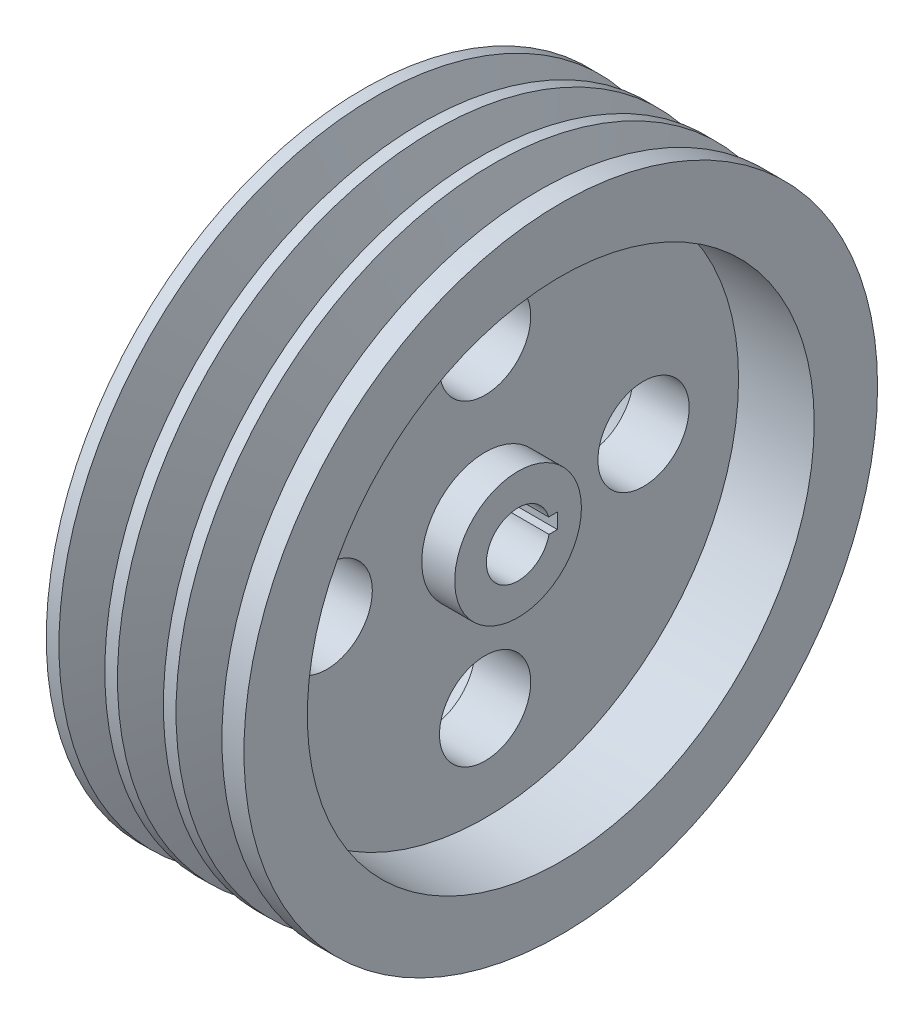
ISO-10303-21;
HEADER;
FILE_DESCRIPTION(('STEP AP214'),'2;1');
FILE_NAME('part.step','',(''),(''),'','','');
FILE_SCHEMA(('AUTOMOTIVE_DESIGN { 1 0 10303 214 1 1 1 1 }'));
ENDSEC;
DATA;
#1=APPLICATION_CONTEXT('core data for automotive mechanical design processes');
#2=APPLICATION_PROTOCOL_DEFINITION('international standard','automotive_design',2000,#1);
#3=PRODUCT_CONTEXT('',#1,'mechanical');
#4=PRODUCT('Part','Part','',(#3));
#5=PRODUCT_RELATED_PRODUCT_CATEGORY('part','',(#4));
#6=PRODUCT_DEFINITION_FORMATION('','',#4);
#7=PRODUCT_DEFINITION_CONTEXT('part definition',#1,'design');
#8=PRODUCT_DEFINITION('design','',#6,#7);
#9=PRODUCT_DEFINITION_SHAPE('','',#8);
#10=(LENGTH_UNIT() NAMED_UNIT(*) SI_UNIT(.MILLI.,.METRE.));
#11=(NAMED_UNIT(*) PLANE_ANGLE_UNIT() SI_UNIT($,.RADIAN.));
#12=(NAMED_UNIT(*) SI_UNIT($,.STERADIAN.) SOLID_ANGLE_UNIT());
#13=UNCERTAINTY_MEASURE_WITH_UNIT(LENGTH_MEASURE(1.E-05),#10,'distance_accuracy_value','');
#14=(GEOMETRIC_REPRESENTATION_CONTEXT(3) GLOBAL_UNCERTAINTY_ASSIGNED_CONTEXT((#13)) GLOBAL_UNIT_ASSIGNED_CONTEXT((#10,
#11,#12)) REPRESENTATION_CONTEXT('',''));
#15=CARTESIAN_POINT('',(0.,0.,0.));
#16=DIRECTION('',(0.,0.,1.));
#17=DIRECTION('',(1.,0.,0.));
#18=AXIS2_PLACEMENT_3D('',#15,#16,#17);
#19=CARTESIAN_POINT('',(-24.,0.,0.));
#20=DIRECTION('',(1.,0.,0.));
#21=DIRECTION('',(0.,0.,-1.));
#22=AXIS2_PLACEMENT_3D('',#19,#20,#21);
#23=PLANE('',#22);
#24=CARTESIAN_POINT('',(-24.,0.,0.));
#25=DIRECTION('',(1.,0.,0.));
#26=DIRECTION('',(0.,0.,-1.));
#27=AXIS2_PLACEMENT_3D('',#24,#25,#26);
#28=CIRCLE('',#27,25.);
#29=CARTESIAN_POINT('',(-24.,0.,-25.));
#30=VERTEX_POINT('',#29);
#31=EDGE_CURVE('E107',#30,#30,#28,.T.);
#32=ORIENTED_EDGE('',*,*,#31,.F.);
#33=EDGE_LOOP('',(#32));
#34=FACE_BOUND('',#33,.T.);
#35=DIRECTION('',(0.,0.,-1.));
#36=VECTOR('',#35,1.);
#37=CARTESIAN_POINT('',(-24.,3.31611385733775,0.));
#38=LINE('',#37,#36);
#39=CARTESIAN_POINT('',(-24.,3.31611385733775,-12.0521113870215));
#40=VERTEX_POINT('',#39);
#41=CARTESIAN_POINT('',(-24.,3.31611385733775,-15.5));
#42=VERTEX_POINT('',#41);
#43=EDGE_CURVE('E105',#40,#42,#38,.T.);
#44=ORIENTED_EDGE('',*,*,#43,.F.);
#45=CARTESIAN_POINT('',(-24.,0.,0.));
#46=DIRECTION('',(1.,0.,0.));
#47=DIRECTION('',(0.,0.,-1.));
#48=AXIS2_PLACEMENT_3D('',#45,#46,#47);
#49=CIRCLE('',#48,12.5);
#50=CARTESIAN_POINT('',(-24.,-2.68388614266225,-12.2084706320335));
#51=VERTEX_POINT('',#50);
#52=EDGE_CURVE('E95',#40,#51,#49,.T.);
#53=ORIENTED_EDGE('',*,*,#52,.T.);
#54=DIRECTION('',(0.,0.,-1.));
#55=VECTOR('',#54,1.);
#56=CARTESIAN_POINT('',(-24.,-2.68388614266225,0.));
#57=LINE('',#56,#55);
#58=CARTESIAN_POINT('',(-24.,-2.68388614266225,-15.5));
#59=VERTEX_POINT('',#58);
#60=EDGE_CURVE('E100',#51,#59,#57,.T.);
#61=ORIENTED_EDGE('',*,*,#60,.T.);
#62=DIRECTION('',(0.,-1.,0.));
#63=VECTOR('',#62,1.);
#64=CARTESIAN_POINT('',(-24.,0.,-15.5));
#65=LINE('',#64,#63);
#66=EDGE_CURVE('E110',#42,#59,#65,.T.);
#67=ORIENTED_EDGE('',*,*,#66,.F.);
#68=EDGE_LOOP('',(#44,#53,#61,#67));
#69=FACE_BOUND('',#68,.T.);
#70=ADVANCED_FACE('F53',(#34,#69),#23,.F.);
#71=CARTESIAN_POINT('',(24.,0.,0.));
#72=DIRECTION('',(1.,0.,0.));
#73=DIRECTION('',(0.,0.,-1.));
#74=AXIS2_PLACEMENT_3D('',#71,#72,#73);
#75=PLANE('',#74);
#76=CARTESIAN_POINT('',(24.,0.,0.));
#77=DIRECTION('',(1.,0.,0.));
#78=DIRECTION('',(0.,0.,-1.));
#79=AXIS2_PLACEMENT_3D('',#76,#77,#78);
#80=CIRCLE('',#79,25.);
#81=CARTESIAN_POINT('',(24.,0.,-25.));
#82=VERTEX_POINT('',#81);
#83=EDGE_CURVE('E112',#82,#82,#80,.T.);
#84=ORIENTED_EDGE('',*,*,#83,.T.);
#85=EDGE_LOOP('',(#84));
#86=FACE_BOUND('',#85,.T.);
#87=CARTESIAN_POINT('',(24.,0.,0.));
#88=DIRECTION('',(1.,0.,0.));
#89=DIRECTION('',(0.,0.,-1.));
#90=AXIS2_PLACEMENT_3D('',#87,#88,#89);
#91=CIRCLE('',#90,12.5);
#92=CARTESIAN_POINT('',(24.,3.31611385733775,-12.0521113870215));
#93=VERTEX_POINT('',#92);
#94=CARTESIAN_POINT('',(24.,-2.68388614266225,-12.2084706320335));
#95=VERTEX_POINT('',#94);
#96=EDGE_CURVE('E189',#93,#95,#91,.T.);
#97=ORIENTED_EDGE('',*,*,#96,.F.);
#98=DIRECTION('',(0.,0.,-1.));
#99=VECTOR('',#98,1.);
#100=CARTESIAN_POINT('',(24.,3.31611385733775,0.));
#101=LINE('',#100,#99);
#102=CARTESIAN_POINT('',(24.,3.31611385733775,-15.5));
#103=VERTEX_POINT('',#102);
#104=EDGE_CURVE('E12',#93,#103,#101,.T.);
#105=ORIENTED_EDGE('',*,*,#104,.T.);
#106=DIRECTION('',(0.,-1.,0.));
#107=VECTOR('',#106,1.);
#108=CARTESIAN_POINT('',(24.,0.,-15.5));
#109=LINE('',#108,#107);
#110=CARTESIAN_POINT('',(24.,-2.68388614266225,-15.5));
#111=VERTEX_POINT('',#110);
#112=EDGE_CURVE('E62',#103,#111,#109,.T.);
#113=ORIENTED_EDGE('',*,*,#112,.T.);
#114=DIRECTION('',(0.,0.,-1.));
#115=VECTOR('',#114,1.);
#116=CARTESIAN_POINT('',(24.,-2.68388614266225,0.));
#117=LINE('',#116,#115);
#118=EDGE_CURVE('E204',#95,#111,#117,.T.);
#119=ORIENTED_EDGE('',*,*,#118,.F.);
#120=EDGE_LOOP('',(#97,#105,#113,#119));
#121=FACE_BOUND('',#120,.T.);
#122=ADVANCED_FACE('F208',(#86,#121),#75,.T.);
#123=CARTESIAN_POINT('',(-37.154392650375,125.,0.));
#124=DIRECTION('',(-1.,0.,0.));
#125=DIRECTION('',(0.,0.,1.));
#126=AXIS2_PLACEMENT_3D('',#123,#124,#125);
#127=PLANE('',#126);
#128=CARTESIAN_POINT('',(-37.154392650375,0.,0.));
#129=DIRECTION('',(-1.,0.,0.));
#130=DIRECTION('',(0.,0.,1.));
#131=AXIS2_PLACEMENT_3D('',#128,#129,#130);
#132=CIRCLE('',#131,100.);
#133=CARTESIAN_POINT('',(-37.154392650375,0.,100.));
#134=VERTEX_POINT('',#133);
#135=EDGE_CURVE('E143',#134,#134,#132,.F.);
#136=ORIENTED_EDGE('',*,*,#135,.T.);
#137=EDGE_LOOP('',(#136));
#138=FACE_BOUND('',#137,.T.);
#139=CARTESIAN_POINT('',(-37.154392650375,0.,0.));
#140=DIRECTION('',(1.,0.,0.));
#141=DIRECTION('',(0.,0.,-1.));
#142=AXIS2_PLACEMENT_3D('',#139,#140,#141);
#143=CIRCLE('',#142,125.);
#144=CARTESIAN_POINT('',(-37.154392650375,0.,-125.));
#145=VERTEX_POINT('',#144);
#146=EDGE_CURVE('E148',#145,#145,#143,.T.);
#147=ORIENTED_EDGE('',*,*,#146,.F.);
#148=EDGE_LOOP('',(#147));
#149=FACE_BOUND('',#148,.T.);
#150=ADVANCED_FACE('F57',(#138,#149),#127,.T.);
#151=CARTESIAN_POINT('',(40.8456073496251,125.,0.));
#152=DIRECTION('',(1.,0.,0.));
#153=DIRECTION('',(0.,0.,-1.));
#154=AXIS2_PLACEMENT_3D('',#151,#152,#153);
#155=PLANE('',#154);
#156=CARTESIAN_POINT('',(40.8456073496251,0.,0.));
#157=DIRECTION('',(1.,0.,0.));
#158=DIRECTION('',(0.,0.,-1.));
#159=AXIS2_PLACEMENT_3D('',#156,#157,#158);
#160=CIRCLE('',#159,100.);
#161=CARTESIAN_POINT('',(40.8456073496251,0.,-100.));
#162=VERTEX_POINT('',#161);
#163=EDGE_CURVE('E144',#162,#162,#160,.T.);
#164=ORIENTED_EDGE('',*,*,#163,.F.);
#165=EDGE_LOOP('',(#164));
#166=FACE_BOUND('',#165,.T.);
#167=CARTESIAN_POINT('',(40.8456073496251,0.,0.));
#168=DIRECTION('',(1.,0.,0.));
#169=DIRECTION('',(0.,0.,-1.));
#170=AXIS2_PLACEMENT_3D('',#167,#168,#169);
#171=CIRCLE('',#170,125.);
#172=CARTESIAN_POINT('',(40.8456073496251,0.,-125.));
#173=VERTEX_POINT('',#172);
#174=EDGE_CURVE('E183',#173,#173,#171,.T.);
#175=ORIENTED_EDGE('',*,*,#174,.T.);
#176=EDGE_LOOP('',(#175));
#177=FACE_BOUND('',#176,.T.);
#178=ADVANCED_FACE('F326',(#166,#177),#155,.T.);
#179=CARTESIAN_POINT('',(491.806779686845,0.,0.));
#180=DIRECTION('',(1.,0.,0.));
#181=DIRECTION('',(0.,0.,-1.));
#182=AXIS2_PLACEMENT_3D('',#179,#180,#181);
#183=CYLINDRICAL_SURFACE('',#182,125.);
#184=CARTESIAN_POINT('',(32.154392650375,0.,0.));
#185=DIRECTION('',(1.,0.,0.));
#186=DIRECTION('',(0.,0.,-1.));
#187=AXIS2_PLACEMENT_3D('',#184,#185,#186);
#188=CIRCLE('',#187,125.);
#189=CARTESIAN_POINT('',(32.154392650375,0.,-125.));
#190=VERTEX_POINT('',#189);
#191=EDGE_CURVE('E185',#190,#190,#188,.T.);
#192=ORIENTED_EDGE('',*,*,#191,.T.);
#193=EDGE_LOOP('',(#192));
#194=FACE_BOUND('',#193,.T.);
#195=ORIENTED_EDGE('',*,*,#174,.F.);
#196=EDGE_LOOP('',(#195));
#197=FACE_BOUND('',#196,.T.);
#198=ADVANCED_FACE('F323',(#194,#197),#183,.T.);
#199=CARTESIAN_POINT('',(32.154392650375,0.,0.));
#200=DIRECTION('',(1.,0.,0.));
#201=DIRECTION('',(0.,0.,-1.));
#202=AXIS2_PLACEMENT_3D('',#199,#200,#201);
#203=CONICAL_SURFACE('',#202,125.,1.22173047639603);
#204=CARTESIAN_POINT('',(25.6029284335833,0.,0.));
#205=DIRECTION('',(1.,0.,0.));
#206=DIRECTION('',(0.,0.,-1.));
#207=AXIS2_PLACEMENT_3D('',#204,#205,#206);
#208=CIRCLE('',#207,107.);
#209=CARTESIAN_POINT('',(25.6029284335833,0.,-107.));
#210=VERTEX_POINT('',#209);
#211=EDGE_CURVE('E178',#210,#210,#208,.T.);
#212=ORIENTED_EDGE('',*,*,#211,.T.);
#213=EDGE_LOOP('',(#212));
#214=FACE_BOUND('',#213,.T.);
#215=ORIENTED_EDGE('',*,*,#191,.F.);
#216=EDGE_LOOP('',(#215));
#217=FACE_BOUND('',#216,.T.);
#218=ADVANCED_FACE('F317',(#214,#217),#203,.T.);
#219=CARTESIAN_POINT('',(491.806779686845,0.,0.));
#220=DIRECTION('',(1.,0.,0.));
#221=DIRECTION('',(0.,0.,-1.));
#222=AXIS2_PLACEMENT_3D('',#219,#220,#221);
#223=CYLINDRICAL_SURFACE('',#222,107.);
#224=CARTESIAN_POINT('',(20.6029284335833,0.,0.));
#225=DIRECTION('',(1.,0.,0.));
#226=DIRECTION('',(0.,0.,-1.));
#227=AXIS2_PLACEMENT_3D('',#224,#225,#226);
#228=CIRCLE('',#227,107.);
#229=CARTESIAN_POINT('',(20.6029284335833,0.,-107.));
#230=VERTEX_POINT('',#229);
#231=EDGE_CURVE('E176',#230,#230,#228,.T.);
#232=ORIENTED_EDGE('',*,*,#231,.T.);
#233=EDGE_LOOP('',(#232));
#234=FACE_BOUND('',#233,.T.);
#235=ORIENTED_EDGE('',*,*,#211,.F.);
#236=EDGE_LOOP('',(#235));
#237=FACE_BOUND('',#236,.T.);
#238=ADVANCED_FACE('F312',(#234,#237),#223,.T.);
#239=CARTESIAN_POINT('',(20.6029284335833,0.,0.));
#240=DIRECTION('',(-1.,0.,0.));
#241=DIRECTION('',(0.,0.,1.));
#242=AXIS2_PLACEMENT_3D('',#239,#240,#241);
#243=CONICAL_SURFACE('',#242,107.,1.22173047639603);
#244=CARTESIAN_POINT('',(14.0514642167917,0.,0.));
#245=DIRECTION('',(1.,0.,0.));
#246=DIRECTION('',(0.,0.,-1.));
#247=AXIS2_PLACEMENT_3D('',#244,#245,#246);
#248=CIRCLE('',#247,125.);
#249=CARTESIAN_POINT('',(14.0514642167917,0.,-125.));
#250=VERTEX_POINT('',#249);
#251=EDGE_CURVE('E174',#250,#250,#248,.T.);
#252=ORIENTED_EDGE('',*,*,#251,.T.);
#253=EDGE_LOOP('',(#252));
#254=FACE_BOUND('',#253,.T.);
#255=ORIENTED_EDGE('',*,*,#231,.F.);
#256=EDGE_LOOP('',(#255));
#257=FACE_BOUND('',#256,.T.);
#258=ADVANCED_FACE('F313',(#254,#257),#243,.T.);
#259=CARTESIAN_POINT('',(491.806779686845,0.,0.));
#260=DIRECTION('',(1.,0.,0.));
#261=DIRECTION('',(0.,0.,-1.));
#262=AXIS2_PLACEMENT_3D('',#259,#260,#261);
#263=CYLINDRICAL_SURFACE('',#262,125.);
#264=CARTESIAN_POINT('',(9.0514642167917,0.,0.));
#265=DIRECTION('',(1.,0.,0.));
#266=DIRECTION('',(0.,0.,-1.));
#267=AXIS2_PLACEMENT_3D('',#264,#265,#266);
#268=CIRCLE('',#267,125.);
#269=CARTESIAN_POINT('',(9.0514642167917,0.,-125.));
#270=VERTEX_POINT('',#269);
#271=EDGE_CURVE('E168',#270,#270,#268,.T.);
#272=ORIENTED_EDGE('',*,*,#271,.T.);
#273=EDGE_LOOP('',(#272));
#274=FACE_BOUND('',#273,.T.);
#275=ORIENTED_EDGE('',*,*,#251,.F.);
#276=EDGE_LOOP('',(#275));
#277=FACE_BOUND('',#276,.T.);
#278=ADVANCED_FACE('F307',(#274,#277),#263,.T.);
#279=CARTESIAN_POINT('',(9.0514642167917,0.,0.));
#280=DIRECTION('',(1.,0.,0.));
#281=DIRECTION('',(0.,0.,-1.));
#282=AXIS2_PLACEMENT_3D('',#279,#280,#281);
#283=CONICAL_SURFACE('',#282,125.,1.22173047639603);
#284=CARTESIAN_POINT('',(2.50000000000006,0.,0.));
#285=DIRECTION('',(1.,0.,0.));
#286=DIRECTION('',(0.,0.,-1.));
#287=AXIS2_PLACEMENT_3D('',#284,#285,#286);
#288=CIRCLE('',#287,107.);
#289=CARTESIAN_POINT('',(2.50000000000006,0.,-107.));
#290=VERTEX_POINT('',#289);
#291=EDGE_CURVE('E170',#290,#290,#288,.T.);
#292=ORIENTED_EDGE('',*,*,#291,.T.);
#293=EDGE_LOOP('',(#292));
#294=FACE_BOUND('',#293,.T.);
#295=ORIENTED_EDGE('',*,*,#271,.F.);
#296=EDGE_LOOP('',(#295));
#297=FACE_BOUND('',#296,.T.);
#298=ADVANCED_FACE('F304',(#294,#297),#283,.T.);
#299=CARTESIAN_POINT('',(491.806779686845,0.,0.));
#300=DIRECTION('',(1.,0.,0.));
#301=DIRECTION('',(0.,0.,-1.));
#302=AXIS2_PLACEMENT_3D('',#299,#300,#301);
#303=CYLINDRICAL_SURFACE('',#302,107.);
#304=CARTESIAN_POINT('',(-2.49999999999995,0.,0.));
#305=DIRECTION('',(1.,0.,0.));
#306=DIRECTION('',(0.,0.,-1.));
#307=AXIS2_PLACEMENT_3D('',#304,#305,#306);
#308=CIRCLE('',#307,107.);
#309=CARTESIAN_POINT('',(-2.49999999999995,0.,-107.));
#310=VERTEX_POINT('',#309);
#311=EDGE_CURVE('E163',#310,#310,#308,.T.);
#312=ORIENTED_EDGE('',*,*,#311,.T.);
#313=EDGE_LOOP('',(#312));
#314=FACE_BOUND('',#313,.T.);
#315=ORIENTED_EDGE('',*,*,#291,.F.);
#316=EDGE_LOOP('',(#315));
#317=FACE_BOUND('',#316,.T.);
#318=ADVANCED_FACE('F298',(#314,#317),#303,.T.);
#319=CARTESIAN_POINT('',(-2.49999999999995,0.,0.));
#320=DIRECTION('',(-1.,0.,0.));
#321=DIRECTION('',(0.,0.,1.));
#322=AXIS2_PLACEMENT_3D('',#319,#320,#321);
#323=CONICAL_SURFACE('',#322,107.,1.22173047639603);
#324=CARTESIAN_POINT('',(-9.05146421679165,0.,0.));
#325=DIRECTION('',(1.,0.,0.));
#326=DIRECTION('',(0.,0.,-1.));
#327=AXIS2_PLACEMENT_3D('',#324,#325,#326);
#328=CIRCLE('',#327,125.);
#329=CARTESIAN_POINT('',(-9.05146421679165,0.,-125.));
#330=VERTEX_POINT('',#329);
#331=EDGE_CURVE('E161',#330,#330,#328,.T.);
#332=ORIENTED_EDGE('',*,*,#331,.T.);
#333=EDGE_LOOP('',(#332));
#334=FACE_BOUND('',#333,.T.);
#335=ORIENTED_EDGE('',*,*,#311,.F.);
#336=EDGE_LOOP('',(#335));
#337=FACE_BOUND('',#336,.T.);
#338=ADVANCED_FACE('F293',(#334,#337),#323,.T.);
#339=CARTESIAN_POINT('',(491.806779686845,0.,0.));
#340=DIRECTION('',(1.,0.,0.));
#341=DIRECTION('',(0.,0.,-1.));
#342=AXIS2_PLACEMENT_3D('',#339,#340,#341);
#343=CYLINDRICAL_SURFACE('',#342,125.);
#344=CARTESIAN_POINT('',(-14.0514642167917,0.,0.));
#345=DIRECTION('',(1.,0.,0.));
#346=DIRECTION('',(0.,0.,-1.));
#347=AXIS2_PLACEMENT_3D('',#344,#345,#346);
#348=CIRCLE('',#347,125.);
#349=CARTESIAN_POINT('',(-14.0514642167917,0.,-125.));
#350=VERTEX_POINT('',#349);
#351=EDGE_CURVE('E158',#350,#350,#348,.T.);
#352=ORIENTED_EDGE('',*,*,#351,.T.);
#353=EDGE_LOOP('',(#352));
#354=FACE_BOUND('',#353,.T.);
#355=ORIENTED_EDGE('',*,*,#331,.F.);
#356=EDGE_LOOP('',(#355));
#357=FACE_BOUND('',#356,.T.);
#358=ADVANCED_FACE('F292',(#354,#357),#343,.T.);
#359=CARTESIAN_POINT('',(-14.0514642167917,0.,0.));
#360=DIRECTION('',(1.,0.,0.));
#361=DIRECTION('',(0.,0.,-1.));
#362=AXIS2_PLACEMENT_3D('',#359,#360,#361);
#363=CONICAL_SURFACE('',#362,125.,1.22173047639603);
#364=CARTESIAN_POINT('',(-20.6029284335833,0.,0.));
#365=DIRECTION('',(1.,0.,0.));
#366=DIRECTION('',(0.,0.,-1.));
#367=AXIS2_PLACEMENT_3D('',#364,#365,#366);
#368=CIRCLE('',#367,107.);
#369=CARTESIAN_POINT('',(-20.6029284335833,0.,-107.));
#370=VERTEX_POINT('',#369);
#371=EDGE_CURVE('E154',#370,#370,#368,.T.);
#372=ORIENTED_EDGE('',*,*,#371,.T.);
#373=EDGE_LOOP('',(#372));
#374=FACE_BOUND('',#373,.T.);
#375=ORIENTED_EDGE('',*,*,#351,.F.);
#376=EDGE_LOOP('',(#375));
#377=FACE_BOUND('',#376,.T.);
#378=ADVANCED_FACE('F287',(#374,#377),#363,.T.);
#379=CARTESIAN_POINT('',(491.806779686845,0.,0.));
#380=DIRECTION('',(1.,0.,0.));
#381=DIRECTION('',(0.,0.,-1.));
#382=AXIS2_PLACEMENT_3D('',#379,#380,#381);
#383=CYLINDRICAL_SURFACE('',#382,107.);
#384=CARTESIAN_POINT('',(-25.6029284335833,0.,0.));
#385=DIRECTION('',(1.,0.,0.));
#386=DIRECTION('',(0.,0.,-1.));
#387=AXIS2_PLACEMENT_3D('',#384,#385,#386);
#388=CIRCLE('',#387,107.);
#389=CARTESIAN_POINT('',(-25.6029284335833,0.,-107.));
#390=VERTEX_POINT('',#389);
#391=EDGE_CURVE('E155',#390,#390,#388,.T.);
#392=ORIENTED_EDGE('',*,*,#391,.T.);
#393=EDGE_LOOP('',(#392));
#394=FACE_BOUND('',#393,.T.);
#395=ORIENTED_EDGE('',*,*,#371,.F.);
#396=EDGE_LOOP('',(#395));
#397=FACE_BOUND('',#396,.T.);
#398=ADVANCED_FACE('F284',(#394,#397),#383,.T.);
#399=CARTESIAN_POINT('',(-25.6029284335833,0.,0.));
#400=DIRECTION('',(-1.,0.,0.));
#401=DIRECTION('',(0.,0.,1.));
#402=AXIS2_PLACEMENT_3D('',#399,#400,#401);
#403=CONICAL_SURFACE('',#402,107.,1.22173047639603);
#404=CARTESIAN_POINT('',(-32.154392650375,0.,0.));
#405=DIRECTION('',(1.,0.,0.));
#406=DIRECTION('',(0.,0.,-1.));
#407=AXIS2_PLACEMENT_3D('',#404,#405,#406);
#408=CIRCLE('',#407,125.);
#409=CARTESIAN_POINT('',(-32.154392650375,0.,-125.));
#410=VERTEX_POINT('',#409);
#411=EDGE_CURVE('E149',#410,#410,#408,.T.);
#412=ORIENTED_EDGE('',*,*,#411,.T.);
#413=EDGE_LOOP('',(#412));
#414=FACE_BOUND('',#413,.T.);
#415=ORIENTED_EDGE('',*,*,#391,.F.);
#416=EDGE_LOOP('',(#415));
#417=FACE_BOUND('',#416,.T.);
#418=ADVANCED_FACE('F276',(#414,#417),#403,.T.);
#419=CARTESIAN_POINT('',(491.806779686845,0.,0.));
#420=DIRECTION('',(1.,0.,0.));
#421=DIRECTION('',(0.,0.,-1.));
#422=AXIS2_PLACEMENT_3D('',#419,#420,#421);
#423=CYLINDRICAL_SURFACE('',#422,125.);
#424=ORIENTED_EDGE('',*,*,#146,.T.);
#425=EDGE_LOOP('',(#424));
#426=FACE_BOUND('',#425,.T.);
#427=ORIENTED_EDGE('',*,*,#411,.F.);
#428=EDGE_LOOP('',(#427));
#429=FACE_BOUND('',#428,.T.);
#430=ADVANCED_FACE('F274',(#426,#429),#423,.T.);
#431=CARTESIAN_POINT('',(11.,0.,0.));
#432=DIRECTION('',(1.,0.,0.));
#433=DIRECTION('',(0.,0.,-1.));
#434=AXIS2_PLACEMENT_3D('',#431,#432,#433);
#435=CYLINDRICAL_SURFACE('',#434,100.);
#436=ORIENTED_EDGE('',*,*,#163,.T.);
#437=EDGE_LOOP('',(#436));
#438=FACE_BOUND('',#437,.T.);
#439=CARTESIAN_POINT('',(11.,0.,0.));
#440=DIRECTION('',(1.,0.,0.));
#441=DIRECTION('',(0.,0.,-1.));
#442=AXIS2_PLACEMENT_3D('',#439,#440,#441);
#443=CIRCLE('',#442,100.);
#444=CARTESIAN_POINT('',(11.,0.,-100.));
#445=VERTEX_POINT('',#444);
#446=EDGE_CURVE('E142',#445,#445,#443,.T.);
#447=ORIENTED_EDGE('',*,*,#446,.F.);
#448=EDGE_LOOP('',(#447));
#449=FACE_BOUND('',#448,.T.);
#450=ADVANCED_FACE('F271',(#438,#449),#435,.F.);
#451=CARTESIAN_POINT('',(11.,0.,0.));
#452=DIRECTION('',(1.,0.,0.));
#453=DIRECTION('',(0.,0.,-1.));
#454=AXIS2_PLACEMENT_3D('',#451,#452,#453);
#455=PLANE('',#454);
#456=CARTESIAN_POINT('',(11.,0.,0.));
#457=DIRECTION('',(1.,0.,0.));
#458=DIRECTION('',(0.,0.,-1.));
#459=AXIS2_PLACEMENT_3D('',#456,#457,#458);
#460=CIRCLE('',#459,25.);
#461=CARTESIAN_POINT('',(11.,0.,-25.));
#462=VERTEX_POINT('',#461);
#463=EDGE_CURVE('E118',#462,#462,#460,.F.);
#464=ORIENTED_EDGE('',*,*,#463,.T.);
#465=EDGE_LOOP('',(#464));
#466=FACE_BOUND('',#465,.T.);
#467=CARTESIAN_POINT('',(11.,0.,-62.5));
#468=DIRECTION('',(1.,0.,0.));
#469=DIRECTION('',(0.,0.,-1.));
#470=AXIS2_PLACEMENT_3D('',#467,#468,#469);
#471=CIRCLE('',#470,18.);
#472=CARTESIAN_POINT('',(11.,0.,-80.5));
#473=VERTEX_POINT('',#472);
#474=EDGE_CURVE('E135',#473,#473,#471,.T.);
#475=ORIENTED_EDGE('',*,*,#474,.F.);
#476=EDGE_LOOP('',(#475));
#477=FACE_BOUND('',#476,.T.);
#478=CARTESIAN_POINT('',(11.,-62.5,2.18217583677696E-13));
#479=DIRECTION('',(1.,0.,0.));
#480=DIRECTION('',(0.,0.,-1.));
#481=AXIS2_PLACEMENT_3D('',#478,#479,#480);
#482=CIRCLE('',#481,18.);
#483=CARTESIAN_POINT('',(11.,-62.5,-17.9999999999998));
#484=VERTEX_POINT('',#483);
#485=EDGE_CURVE('E131',#484,#484,#482,.T.);
#486=ORIENTED_EDGE('',*,*,#485,.F.);
#487=EDGE_LOOP('',(#486));
#488=FACE_BOUND('',#487,.T.);
#489=CARTESIAN_POINT('',(11.,4.36435167355392E-13,62.5));
#490=DIRECTION('',(1.,0.,0.));
#491=DIRECTION('',(0.,0.,-1.));
#492=AXIS2_PLACEMENT_3D('',#489,#490,#491);
#493=CIRCLE('',#492,18.);
#494=CARTESIAN_POINT('',(11.,4.36435167355392E-13,44.5));
#495=VERTEX_POINT('',#494);
#496=EDGE_CURVE('E130',#495,#495,#493,.T.);
#497=ORIENTED_EDGE('',*,*,#496,.F.);
#498=EDGE_LOOP('',(#497));
#499=FACE_BOUND('',#498,.T.);
#500=CARTESIAN_POINT('',(11.,62.5,-6.54652751033088E-13));
#501=DIRECTION('',(1.,0.,0.));
#502=DIRECTION('',(0.,0.,-1.));
#503=AXIS2_PLACEMENT_3D('',#500,#501,#502);
#504=CIRCLE('',#503,18.);
#505=CARTESIAN_POINT('',(11.,62.5,-18.0000000000007));
#506=VERTEX_POINT('',#505);
#507=EDGE_CURVE('E124',#506,#506,#504,.T.);
#508=ORIENTED_EDGE('',*,*,#507,.F.);
#509=EDGE_LOOP('',(#508));
#510=FACE_BOUND('',#509,.T.);
#511=ORIENTED_EDGE('',*,*,#446,.T.);
#512=EDGE_LOOP('',(#511));
#513=FACE_BOUND('',#512,.T.);
#514=ADVANCED_FACE('F270',(#466,#477,#488,#499,#510,#513),#455,.T.);
#515=CARTESIAN_POINT('',(-11.,0.,0.));
#516=DIRECTION('',(-1.,0.,0.));
#517=DIRECTION('',(0.,0.,1.));
#518=AXIS2_PLACEMENT_3D('',#515,#516,#517);
#519=CYLINDRICAL_SURFACE('',#518,100.);
#520=ORIENTED_EDGE('',*,*,#135,.F.);
#521=EDGE_LOOP('',(#520));
#522=FACE_BOUND('',#521,.T.);
#523=CARTESIAN_POINT('',(-11.,0.,0.));
#524=DIRECTION('',(1.,0.,0.));
#525=DIRECTION('',(0.,0.,-1.));
#526=AXIS2_PLACEMENT_3D('',#523,#524,#525);
#527=CIRCLE('',#526,100.);
#528=CARTESIAN_POINT('',(-11.,0.,-100.));
#529=VERTEX_POINT('',#528);
#530=EDGE_CURVE('E139',#529,#529,#527,.T.);
#531=ORIENTED_EDGE('',*,*,#530,.T.);
#532=EDGE_LOOP('',(#531));
#533=FACE_BOUND('',#532,.T.);
#534=ADVANCED_FACE('F263',(#522,#533),#519,.F.);
#535=CARTESIAN_POINT('',(-11.,0.,0.));
#536=DIRECTION('',(-1.,0.,0.));
#537=DIRECTION('',(0.,0.,-1.));
#538=AXIS2_PLACEMENT_3D('',#535,#536,#537);
#539=PLANE('',#538);
#540=CARTESIAN_POINT('',(-11.,0.,0.));
#541=DIRECTION('',(-1.,0.,0.));
#542=DIRECTION('',(0.,0.,1.));
#543=AXIS2_PLACEMENT_3D('',#540,#541,#542);
#544=CIRCLE('',#543,25.);
#545=CARTESIAN_POINT('',(-11.,0.,25.));
#546=VERTEX_POINT('',#545);
#547=EDGE_CURVE('E117',#546,#546,#544,.F.);
#548=ORIENTED_EDGE('',*,*,#547,.T.);
#549=EDGE_LOOP('',(#548));
#550=FACE_BOUND('',#549,.T.);
#551=CARTESIAN_POINT('',(-11.,0.,-62.5));
#552=DIRECTION('',(-1.,0.,0.));
#553=DIRECTION('',(0.,0.,1.));
#554=AXIS2_PLACEMENT_3D('',#551,#552,#553);
#555=CIRCLE('',#554,18.);
#556=CARTESIAN_POINT('',(-11.,0.,-44.5));
#557=VERTEX_POINT('',#556);
#558=EDGE_CURVE('E133',#557,#557,#555,.T.);
#559=ORIENTED_EDGE('',*,*,#558,.F.);
#560=EDGE_LOOP('',(#559));
#561=FACE_BOUND('',#560,.T.);
#562=CARTESIAN_POINT('',(-11.,-62.5,2.18217583677696E-13));
#563=DIRECTION('',(-1.,0.,0.));
#564=DIRECTION('',(0.,0.,1.));
#565=AXIS2_PLACEMENT_3D('',#562,#563,#564);
#566=CIRCLE('',#565,18.);
#567=CARTESIAN_POINT('',(-11.,-62.5,18.0000000000002));
#568=VERTEX_POINT('',#567);
#569=EDGE_CURVE('E128',#568,#568,#566,.T.);
#570=ORIENTED_EDGE('',*,*,#569,.F.);
#571=EDGE_LOOP('',(#570));
#572=FACE_BOUND('',#571,.T.);
#573=CARTESIAN_POINT('',(-11.,4.36435167355392E-13,62.5));
#574=DIRECTION('',(-1.,0.,0.));
#575=DIRECTION('',(0.,0.,1.));
#576=AXIS2_PLACEMENT_3D('',#573,#574,#575);
#577=CIRCLE('',#576,18.);
#578=CARTESIAN_POINT('',(-11.,4.36435167355392E-13,80.5));
#579=VERTEX_POINT('',#578);
#580=EDGE_CURVE('E127',#579,#579,#577,.T.);
#581=ORIENTED_EDGE('',*,*,#580,.F.);
#582=EDGE_LOOP('',(#581));
#583=FACE_BOUND('',#582,.T.);
#584=CARTESIAN_POINT('',(-11.,62.5,-6.54652751033088E-13));
#585=DIRECTION('',(-1.,0.,0.));
#586=DIRECTION('',(0.,0.,1.));
#587=AXIS2_PLACEMENT_3D('',#584,#585,#586);
#588=CIRCLE('',#587,18.);
#589=CARTESIAN_POINT('',(-11.,62.5,17.9999999999993));
#590=VERTEX_POINT('',#589);
#591=EDGE_CURVE('E122',#590,#590,#588,.T.);
#592=ORIENTED_EDGE('',*,*,#591,.F.);
#593=EDGE_LOOP('',(#592));
#594=FACE_BOUND('',#593,.T.);
#595=ORIENTED_EDGE('',*,*,#530,.F.);
#596=EDGE_LOOP('',(#595));
#597=FACE_BOUND('',#596,.T.);
#598=ADVANCED_FACE('F259',(#550,#561,#572,#583,#594,#597),#539,.T.);
#599=CARTESIAN_POINT('',(-50.,62.5,-6.54652751033088E-13));
#600=DIRECTION('',(1.,0.,0.));
#601=DIRECTION('',(0.,0.,-1.));
#602=AXIS2_PLACEMENT_3D('',#599,#600,#601);
#603=CYLINDRICAL_SURFACE('',#602,18.);
#604=ORIENTED_EDGE('',*,*,#507,.T.);
#605=EDGE_LOOP('',(#604));
#606=FACE_BOUND('',#605,.T.);
#607=ORIENTED_EDGE('',*,*,#591,.T.);
#608=EDGE_LOOP('',(#607));
#609=FACE_BOUND('',#608,.T.);
#610=ADVANCED_FACE('F254',(#606,#609),#603,.F.);
#611=CARTESIAN_POINT('',(-50.,4.36435167355392E-13,62.5));
#612=DIRECTION('',(1.,0.,0.));
#613=DIRECTION('',(0.,0.,-1.));
#614=AXIS2_PLACEMENT_3D('',#611,#612,#613);
#615=CYLINDRICAL_SURFACE('',#614,18.);
#616=ORIENTED_EDGE('',*,*,#496,.T.);
#617=EDGE_LOOP('',(#616));
#618=FACE_BOUND('',#617,.T.);
#619=ORIENTED_EDGE('',*,*,#580,.T.);
#620=EDGE_LOOP('',(#619));
#621=FACE_BOUND('',#620,.T.);
#622=ADVANCED_FACE('F253',(#618,#621),#615,.F.);
#623=CARTESIAN_POINT('',(-50.,-62.5,2.18217583677696E-13));
#624=DIRECTION('',(1.,0.,0.));
#625=DIRECTION('',(0.,0.,-1.));
#626=AXIS2_PLACEMENT_3D('',#623,#624,#625);
#627=CYLINDRICAL_SURFACE('',#626,18.);
#628=ORIENTED_EDGE('',*,*,#485,.T.);
#629=EDGE_LOOP('',(#628));
#630=FACE_BOUND('',#629,.T.);
#631=ORIENTED_EDGE('',*,*,#569,.T.);
#632=EDGE_LOOP('',(#631));
#633=FACE_BOUND('',#632,.T.);
#634=ADVANCED_FACE('F247',(#630,#633),#627,.F.);
#635=CARTESIAN_POINT('',(-50.,0.,-62.5));
#636=DIRECTION('',(1.,0.,0.));
#637=DIRECTION('',(0.,0.,-1.));
#638=AXIS2_PLACEMENT_3D('',#635,#636,#637);
#639=CYLINDRICAL_SURFACE('',#638,18.);
#640=ORIENTED_EDGE('',*,*,#474,.T.);
#641=EDGE_LOOP('',(#640));
#642=FACE_BOUND('',#641,.T.);
#643=ORIENTED_EDGE('',*,*,#558,.T.);
#644=EDGE_LOOP('',(#643));
#645=FACE_BOUND('',#644,.T.);
#646=ADVANCED_FACE('F244',(#642,#645),#639,.F.);
#647=CARTESIAN_POINT('',(24.,0.,0.));
#648=DIRECTION('',(-1.,0.,0.));
#649=DIRECTION('',(0.,0.,1.));
#650=AXIS2_PLACEMENT_3D('',#647,#648,#649);
#651=CYLINDRICAL_SURFACE('',#650,25.);
#652=ORIENTED_EDGE('',*,*,#547,.F.);
#653=EDGE_LOOP('',(#652));
#654=FACE_BOUND('',#653,.T.);
#655=ORIENTED_EDGE('',*,*,#31,.T.);
#656=EDGE_LOOP('',(#655));
#657=FACE_BOUND('',#656,.T.);
#658=ADVANCED_FACE('F239',(#654,#657),#651,.T.);
#659=ORIENTED_EDGE('',*,*,#463,.F.);
#660=EDGE_LOOP('',(#659));
#661=FACE_BOUND('',#660,.T.);
#662=ORIENTED_EDGE('',*,*,#83,.F.);
#663=EDGE_LOOP('',(#662));
#664=FACE_BOUND('',#663,.T.);
#665=ADVANCED_FACE('F242',(#661,#664),#651,.T.);
#666=CARTESIAN_POINT('',(-100.,3.31611385733775,-4.62011831581656));
#667=DIRECTION('',(0.,-1.,0.));
#668=DIRECTION('',(0.,0.,-1.));
#669=AXIS2_PLACEMENT_3D('',#666,#667,#668);
#670=PLANE('',#669);
#671=ORIENTED_EDGE('',*,*,#43,.T.);
#672=DIRECTION('',(1.,0.,0.));
#673=VECTOR('',#672,1.);
#674=CARTESIAN_POINT('',(-100.,3.31611385733775,-15.5));
#675=LINE('',#674,#673);
#676=EDGE_CURVE('E215',#42,#103,#675,.T.);
#677=ORIENTED_EDGE('',*,*,#676,.T.);
#678=ORIENTED_EDGE('',*,*,#104,.F.);
#679=DIRECTION('',(1.,0.,0.));
#680=VECTOR('',#679,1.);
#681=CARTESIAN_POINT('',(-100.,3.31611385733775,-12.0521113870215));
#682=LINE('',#681,#680);
#683=EDGE_CURVE('E74',#40,#93,#682,.T.);
#684=ORIENTED_EDGE('',*,*,#683,.F.);
#685=EDGE_LOOP('',(#671,#677,#678,#684));
#686=FACE_BOUND('',#685,.T.);
#687=ADVANCED_FACE('F99',(#686),#670,.T.);
#688=CARTESIAN_POINT('',(-100.,3.31611385733775,-15.5));
#689=DIRECTION('',(0.,0.,1.));
#690=DIRECTION('',(1.,0.,0.));
#691=AXIS2_PLACEMENT_3D('',#688,#689,#690);
#692=PLANE('',#691);
#693=ORIENTED_EDGE('',*,*,#66,.T.);
#694=DIRECTION('',(1.,0.,0.));
#695=VECTOR('',#694,1.);
#696=CARTESIAN_POINT('',(-100.,-2.68388614266225,-15.5));
#697=LINE('',#696,#695);
#698=EDGE_CURVE('E212',#59,#111,#697,.T.);
#699=ORIENTED_EDGE('',*,*,#698,.T.);
#700=ORIENTED_EDGE('',*,*,#112,.F.);
#701=ORIENTED_EDGE('',*,*,#676,.F.);
#702=EDGE_LOOP('',(#693,#699,#700,#701));
#703=FACE_BOUND('',#702,.T.);
#704=ADVANCED_FACE('F211',(#703),#692,.T.);
#705=CARTESIAN_POINT('',(-100.,-2.68388614266225,-4.62011831581656));
#706=DIRECTION('',(0.,-1.,0.));
#707=DIRECTION('',(0.,0.,-1.));
#708=AXIS2_PLACEMENT_3D('',#705,#706,#707);
#709=PLANE('',#708);
#710=DIRECTION('',(1.,0.,0.));
#711=VECTOR('',#710,1.);
#712=CARTESIAN_POINT('',(-100.,-2.68388614266225,-12.2084706320335));
#713=LINE('',#712,#711);
#714=EDGE_CURVE('E68',#51,#95,#713,.T.);
#715=ORIENTED_EDGE('',*,*,#714,.T.);
#716=ORIENTED_EDGE('',*,*,#118,.T.);
#717=ORIENTED_EDGE('',*,*,#698,.F.);
#718=ORIENTED_EDGE('',*,*,#60,.F.);
#719=EDGE_LOOP('',(#715,#716,#717,#718));
#720=FACE_BOUND('',#719,.T.);
#721=ADVANCED_FACE('F218',(#720),#709,.F.);
#722=CARTESIAN_POINT('',(-100.,0.,0.));
#723=DIRECTION('',(1.,0.,0.));
#724=DIRECTION('',(0.,0.,-1.));
#725=AXIS2_PLACEMENT_3D('',#722,#723,#724);
#726=CYLINDRICAL_SURFACE('',#725,12.5);
#727=ORIENTED_EDGE('',*,*,#683,.T.);
#728=ORIENTED_EDGE('',*,*,#96,.T.);
#729=ORIENTED_EDGE('',*,*,#714,.F.);
#730=ORIENTED_EDGE('',*,*,#52,.F.);
#731=EDGE_LOOP('',(#727,#728,#729,#730));
#732=FACE_BOUND('',#731,.T.);
#733=ADVANCED_FACE('F91',(#732),#726,.F.);
#734=CLOSED_SHELL('',(#70,#122,#150,#178,#198,#218,#238,#258,#278,#298,#318,#338,#358,#378,#398,
#418,#430,#450,#514,#534,#598,#610,#622,#634,#646,#658,#665,#687,#704,#721,#733));
#735=MANIFOLD_SOLID_BREP('B2',#734);
#736=ADVANCED_BREP_SHAPE_REPRESENTATION('',(#18,#735),#14);
#737=SHAPE_DEFINITION_REPRESENTATION(#9,#736);
ENDSEC;
END-ISO-10303-21;
